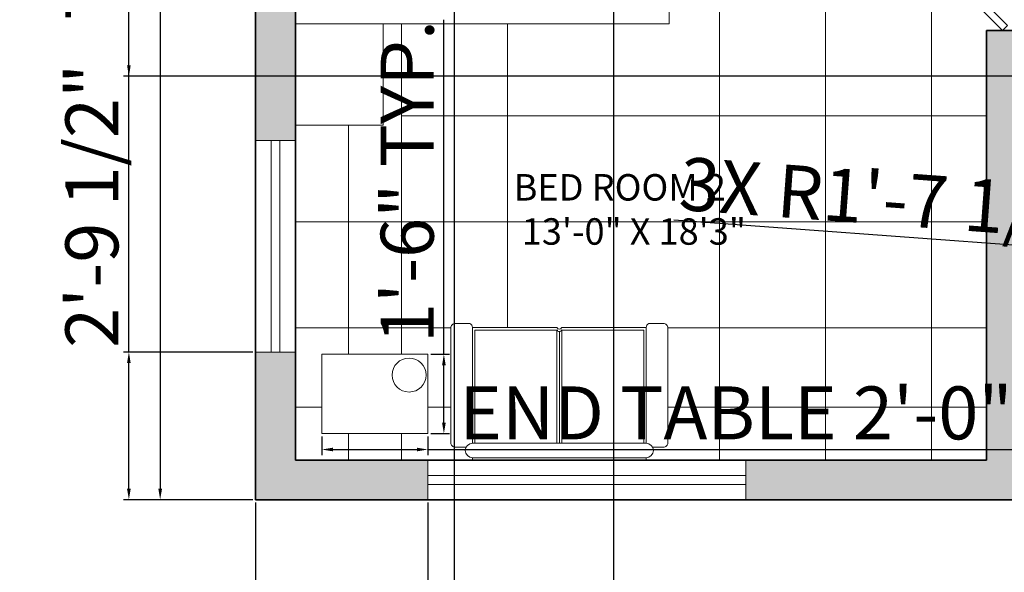
# Model space of a CAD drawing. Units: millimetres. Extents: x 542930 to 543750, y 628093 to 628738.
# Tile 2 of 14: x 542930 to 543153, y 628237 to 628363. Entities that reach past the tile are written whole.
import ezdxf

# ---------------------------------------------------------------- set-up
doc = ezdxf.new("R2010")
doc.units = ezdxf.units.MM
for name, color, linetype, lineweight in [('A-ANNO-DIMS', 2, 'Continuous', 18), ('A-FURN', 8, 'Continuous', 18), ('A-WALL', 7, 'Continuous', 35), ('DOORS', 30, 'Continuous', 18), ('WINDOW', 70, 'Continuous', 18)]:
    doc.layers.add(name, color=color, linetype=linetype, lineweight=lineweight)
for name, color, linetype, lineweight, true_color in [('A-AREA-IDEN', 40, 'Continuous', 18, 0xf8d731), ('A-FLOR-PATT', 241, 'Continuous', 13, 0xf7abae), ('A-WALL-PATT', 251, 'Continuous', 13, 0x636466)]:
    doc.layers.add(name, color=color, linetype=linetype, lineweight=lineweight, true_color=true_color)
doc.styles.get("Standard").update_dxf_attribs({"font": 'arial.ttf'})
doc.dimstyles.new('ISO-25', dxfattribs={"dimtxt": 12, "dimasz": 2.5, "dimexe": 1.25, "dimexo": 0.625, "dimtad": 1, "dimdec": 0, "dimlunit": 3, "dimtxsty": 'Standard', "dimcen": 2.5, "dimadec": 0, "dimazin": 0, "dimtfac": 1, "dimtdec": 0, "dimtmove": 0, "dimatfit": 3, "dimfxl": 1, "dimarcsym": 0})

# ---------------------------------------------------------------- blocks, each defined once
blk = doc.blocks.new('*U4')
for p, q in [((0, 0), (0, -6)), ((40, 0), (40, -6))]:
    blk.add_line(p, q)
blk.add_lwpolyline([(0, 0), (28.28, 28.28), (29.52, 27.05), (1.24, -1.24)], close=True)
blk.add_arc((0, 0), 40, 0, 45)
blk = doc.blocks.new('sofa')
for p, q in [((543001.62, 628230.38), (543001.62, 628182.38)), ((543010.62, 628230.38), (543045.62, 628230.38)), ((543045.62, 628229.38), (543045.62, 628182.38)), ((543046.62, 628228.78), (543046.62, 628182.38)), ((543091.62, 628230.38), (543091.62, 628182.38)), ((543010.62, 628176.38), (543082.62, 628176.38))]:
    blk.add_line(p, q)
for points in [[(543009.53, 628232.06), (543003.46, 628232.06, 0.414214), (543001.62, 628230.23)], [(543045.62, 628230.38, 0.623864), (543047.62, 628230.38), (543082.62, 628230.38), (543082.62, 628182.38), (543010.62, 628182.38), (543010.62, 628230.38, 0.297291), (543009.53, 628232.06)], [(543083.72, 628232.06, 0.297291), (543082.62, 628230.38), (543082.62, 628182.38)], [(543091.62, 628230.23, 0.414214), (543089.79, 628232.06), (543083.72, 628232.06)], [(543001.62, 628182.54, 0.414214), (543003.46, 628180.7), (543007.93, 628180.7)], [(543082.62, 628182.38, -1), (543082.62, 628176.38), (543082.62, 628175.38), (543010.62, 628175.38), (543010.62, 628176.38, -1), (543010.62, 628182.38)], [(543085.32, 628180.7), (543089.79, 628180.7, 0.414214), (543091.62, 628182.54)]]:
    blk.add_lwpolyline(points, format="xyb")
for points in [[(543011.62, 628182.38), (543011.62, 628229.38), (543045.62, 628229.38), (543045.62, 628229.4)], [(543047.62, 628182.38), (543047.62, 628229.38), (543047.62, 628229.4)], [(543047.62, 628229.38), (543081.62, 628229.38), (543081.62, 628182.38)]]:
    blk.add_lwpolyline(points)
blk.add_arc((543046.62, 628229.89), 1.11, 206.0829, 333.9171)
blk = doc.blocks.new('*D20')
at = {"layer": 'A-ANNO-DIMS', "color": 0, "lineweight": -2, "transparency": 16777216}
for p, q in [((542983.04, 628589.83), (542960.8, 628589.83)), ((542962.05, 628587.33), (542962.05, 628256.33)), ((542983.04, 628253.83), (542960.8, 628253.83))]:
    blk.add_line(p, q, dxfattribs=at)
at = {"layer": 'A-ANNO-DIMS', "color": 0, "transparency": 16777216}
for points in [[(542961.64, 628587.33), (542962.47, 628587.33), (542962.05, 628589.83)], [(542961.64, 628256.33), (542962.47, 628256.33), (542962.05, 628253.83)]]:
    blk.add_solid(points, dxfattribs=at)
at = {"layer": 'Defpoints', "color": 0, "transparency": 16777216}
for p in [(542983.67, 628589.83), (542962.05, 628253.83), (542983.67, 628253.83)]:
    blk.add_point(p, dxfattribs=at)
at = {"layer": 'A-ANNO-DIMS', "color": 0, "transparency": 16777216, "insert": (542955.3, 628421.83), "char_height": 12, "attachment_point": 5, "rotation": 90}
blk.add_mtext("28'", dxfattribs=at)
blk = doc.blocks.new('BEDROOM-END-TABLE')
for p, q in [((0, 0), (0, 18)), ((24.02, 18), (0, 18)), ((24.02, 0), (24.02, 18)), ((24.02, 0), (0, 0))]:
    blk.add_line(p, q)
blk.add_circle((19.74, 13.28), 3.85)
blk = doc.blocks.new('WIN-BEDROOM-FRONT')
for p, q in [((0, 9), (0, 0)), ((72, 9), (72, 0)), ((0, 5.5), (72, 5.5)), ((0, 3.5), (72, 3.5))]:
    blk.add_line(p, q)
blk = doc.blocks.new('WIN-BEDROOM-SIDE')
for p, q in [((0, 48), (9, 48)), ((3.5, 48), (3.5, 0)), ((5.5, 48), (5.5, 0)), ((0, 0), (9, 0))]:
    blk.add_line(p, q)
blk = doc.blocks.new('*D47')
at = {"layer": 'A-ANNO-DIMS', "color": 0, "lineweight": -2, "transparency": 16777216}
for p, q in [((542998.67, 628268.2), (542998.67, 628263.97)), ((543022.69, 628268.2), (543022.69, 628263.97)), ((543001.17, 628265.22), (543020.19, 628265.22)), ((543022.69, 628265.22), (543196.77, 628265.22))]:
    blk.add_line(p, q, dxfattribs=at)
at = {"layer": 'A-ANNO-DIMS', "color": 0, "transparency": 16777216}
for points in [[(543001.17, 628265.64), (543001.17, 628264.81), (542998.67, 628265.22)], [(543020.19, 628265.64), (543020.19, 628264.81), (543022.69, 628265.22)]]:
    blk.add_solid(points, dxfattribs=at)
at = {"layer": 'Defpoints', "color": 0, "transparency": 16777216}
for p in [(542998.67, 628268.83), (543022.69, 628268.83), (543022.69, 628265.22)]:
    blk.add_point(p, dxfattribs=at)
at = {"layer": 'A-ANNO-DIMS', "color": 0, "transparency": 16777216, "insert": (543110.98, 628271.97), "char_height": 12, "attachment_point": 5}
blk.add_mtext('END TABLE 2\'-0" TYP.', dxfattribs=at)
blk = doc.blocks.new('*D48')
at = {"layer": 'A-ANNO-DIMS', "color": 0, "lineweight": -2, "transparency": 16777216}
for p, q in [((543026.29, 628286.83), (543026.29, 628362.59)), ((543023.31, 628286.83), (543027.54, 628286.83)), ((543026.29, 628271.33), (543026.29, 628284.33)), ((543023.31, 628268.83), (543027.54, 628268.83))]:
    blk.add_line(p, q, dxfattribs=at)
at = {"layer": 'A-ANNO-DIMS', "color": 0, "transparency": 16777216}
for points in [[(543025.88, 628284.33), (543026.71, 628284.33), (543026.29, 628286.83)], [(543025.88, 628271.33), (543026.71, 628271.33), (543026.29, 628268.83)]]:
    blk.add_solid(points, dxfattribs=at)
at = {"layer": 'Defpoints', "color": 0, "transparency": 16777216}
for p in [(543022.69, 628286.83), (543026.29, 628286.83), (543022.69, 628268.83)]:
    blk.add_point(p, dxfattribs=at)
at = {"layer": 'A-ANNO-DIMS', "color": 0, "transparency": 16777216, "insert": (543019.54, 628325.96), "char_height": 12, "attachment_point": 5, "rotation": 90}
blk.add_mtext('1\'-6" TYP.', dxfattribs=at)
blk = doc.blocks.new('*D62')
at = {"layer": 'A-ANNO-DIMS', "color": 0, "lineweight": -2, "transparency": 16777216}
for p, q in [((542983.67, 628253.2), (542983.67, 628103.84)), ((543022.69, 628253.2), (543022.69, 628103.84)), ((542986.17, 628105.09), (543020.19, 628105.09))]:
    blk.add_line(p, q, dxfattribs=at)
at = {"layer": 'A-ANNO-DIMS', "color": 0, "transparency": 16777216}
for points in [[(542986.17, 628105.5), (542986.17, 628104.67), (542983.67, 628105.09)], [(543020.19, 628105.5), (543020.19, 628104.67), (543022.69, 628105.09)]]:
    blk.add_solid(points, dxfattribs=at)
at = {"layer": 'Defpoints', "color": 0, "transparency": 16777216}
for p in [(542983.67, 628253.83), (543022.69, 628253.83), (543022.69, 628105.09)]:
    blk.add_point(p, dxfattribs=at)
at = {"layer": 'A-ANNO-DIMS', "color": 0, "transparency": 16777216, "insert": (543003.18, 628111.84), "char_height": 12, "attachment_point": 5}
blk.add_mtext('3\'-3"', dxfattribs=at)
blk = doc.blocks.new('*D64')
at = {"layer": 'A-ANNO-DIMS', "color": 0, "lineweight": -2, "transparency": 16777216}
for p, q in [((542954.97, 628287.3), (542954.97, 628351.12)), ((542983.04, 628287.3), (542953.72, 628287.3)), ((542954.97, 628256.33), (542954.97, 628284.8)), ((542983.04, 628253.83), (542953.72, 628253.83))]:
    blk.add_line(p, q, dxfattribs=at)
at = {"layer": 'A-ANNO-DIMS', "color": 0, "transparency": 16777216}
for points in [[(542954.55, 628284.8), (542955.38, 628284.8), (542954.97, 628287.3)], [(542954.55, 628256.33), (542955.38, 628256.33), (542954.97, 628253.83)]]:
    blk.add_solid(points, dxfattribs=at)
at = {"layer": 'Defpoints', "color": 0, "transparency": 16777216}
for p in [(542954.97, 628287.3), (542983.67, 628287.3), (542983.67, 628253.83)]:
    blk.add_point(p, dxfattribs=at)
at = {"layer": 'A-ANNO-DIMS', "color": 0, "transparency": 16777216, "insert": (542948.14, 628320.46), "char_height": 12, "attachment_point": 5, "rotation": 90}
blk.add_mtext('2\'-9 1/2"', dxfattribs=at)
blk = doc.blocks.new('*D75')
at = {"layer": 'A-ANNO-DIMS', "color": 0, "lineweight": -2, "transparency": 16777216}
for p, q in [((543324.54, 628439.36), (542953.72, 628439.36)), ((542954.97, 628352.33), (542954.97, 628436.86)), ((543324.54, 628349.83), (542953.72, 628349.83))]:
    blk.add_line(p, q, dxfattribs=at)
at = {"layer": 'A-ANNO-DIMS', "color": 0, "transparency": 16777216}
for points in [[(542954.55, 628436.86), (542955.38, 628436.86), (542954.97, 628439.36)], [(542954.55, 628352.33), (542955.38, 628352.33), (542954.97, 628349.83)]]:
    blk.add_solid(points, dxfattribs=at)
at = {"layer": 'Defpoints', "color": 0, "transparency": 16777216}
for p in [(542954.97, 628439.36), (543325.17, 628439.36), (543325.17, 628349.83)]:
    blk.add_point(p, dxfattribs=at)
at = {"layer": 'A-ANNO-DIMS', "color": 0, "transparency": 16777216, "insert": (542948.14, 628394.6), "char_height": 12, "attachment_point": 5, "rotation": 90}
blk.add_mtext('7\'-5 1/2"', dxfattribs=at)
blk = doc.blocks.new('*D85')
at = {"layer": 'A-ANNO-DIMS', "color": 0, "lineweight": -2, "transparency": 16777216}
for p, q in [((543028.62, 628481.2), (543028.62, 628103.84)), ((543064.67, 628481.2), (543064.67, 628103.84)), ((543031.12, 628105.09), (543062.17, 628105.09))]:
    blk.add_line(p, q, dxfattribs=at)
at = {"layer": 'A-ANNO-DIMS', "color": 0, "transparency": 16777216}
for points in [[(543031.12, 628105.5), (543031.12, 628104.67), (543028.62, 628105.09)], [(543062.17, 628105.5), (543062.17, 628104.67), (543064.67, 628105.09)]]:
    blk.add_solid(points, dxfattribs=at)
at = {"layer": 'Defpoints', "color": 0, "transparency": 16777216}
for p in [(543028.62, 628481.83), (543064.67, 628481.83), (543064.67, 628105.09)]:
    blk.add_point(p, dxfattribs=at)
at = {"layer": 'A-ANNO-DIMS', "color": 0, "transparency": 16777216, "insert": (543046.65, 628111.84), "char_height": 12, "attachment_point": 5}
blk.add_mtext('3\'-0"', dxfattribs=at)
blk = doc.blocks.new('*D93')
at = {"layer": 'A-ANNO-DIMS', "color": 0, "lineweight": -2, "transparency": 16777216}
for p, q in [((543078.39, 628317.26), (543178.99, 628309.88)), ((543200.81, 628308.28), (543181.49, 628309.7))]:
    blk.add_line(p, q, dxfattribs=at)
at = {"layer": 'A-ANNO-DIMS', "color": 0, "transparency": 16777216}
blk.add_solid([(543179.02, 628310.3), (543178.96, 628309.46), (543181.49, 628309.7)], dxfattribs=at)
at = {"layer": 'Defpoints', "color": 0, "transparency": 16777216}
for p in [(543181.49, 628309.7), (543200.81, 628308.28)]:
    blk.add_point(p, dxfattribs=at)
at = {"layer": 'A-ANNO-DIMS', "color": 0, "transparency": 16777216, "insert": (543127.94, 628320.48), "char_height": 12, "attachment_point": 5, "rotation": 355.8053}
blk.add_mtext('3X R1\'-7 1/2"', dxfattribs=at)
blk = doc.blocks.new('*D94')
at = {"layer": 'A-ANNO-DIMS', "color": 0, "lineweight": -2, "transparency": 16777216}
for p, q in [((543143.96, 628391.37), (543186.37, 628329.39)), ((543198.34, 628311.9), (543187.78, 628327.33))]:
    blk.add_line(p, q, dxfattribs=at)
at = {"layer": 'A-ANNO-DIMS', "color": 0, "transparency": 16777216}
blk.add_solid([(543186.71, 628329.63), (543186.02, 628329.15), (543187.78, 628327.33)], dxfattribs=at)
at = {"layer": 'Defpoints', "color": 0, "transparency": 16777216}
for p in [(543187.78, 628327.33), (543198.34, 628311.9)]:
    blk.add_point(p, dxfattribs=at)
at = {"layer": 'A-ANNO-DIMS', "color": 0, "transparency": 16777216, "insert": (543170.1, 628365.27), "char_height": 12, "attachment_point": 5, "rotation": 304.3793}
blk.add_mtext('R1\'-6 1/2"', dxfattribs=at)
blk = doc.blocks.new('*D95')
at = {"layer": 'A-ANNO-DIMS', "color": 0, "lineweight": -2, "transparency": 16777216}
for p, q in [((543144.53, 628390.54), (543186.93, 628328.57)), ((543198.34, 628311.9), (543188.34, 628326.5))]:
    blk.add_line(p, q, dxfattribs=at)
at = {"layer": 'A-ANNO-DIMS', "color": 0, "transparency": 16777216}
blk.add_solid([(543187.28, 628328.8), (543186.59, 628328.33), (543188.34, 628326.5)], dxfattribs=at)
at = {"layer": 'Defpoints', "color": 0, "transparency": 16777216}
for p in [(543188.34, 628326.5), (543198.34, 628311.9)]:
    blk.add_point(p, dxfattribs=at)
at = {"layer": 'A-ANNO-DIMS', "color": 0, "transparency": 16777216, "insert": (543170.66, 628364.44), "char_height": 12, "attachment_point": 5, "rotation": 304.3778}
blk.add_mtext('R1\'-5 1/2"', dxfattribs=at)

msp = doc.modelspace()

# ---------------------------------------------------------------- hatches: boundary and pattern name
at = {"layer": 'A-WALL-PATT'}
h = msp.add_hatch(color=256, dxfattribs=at)
h.dxf.hatch_style = 1
h.paths.add_polyline_path([(542992.67, 628481.83), (543028.62, 628481.83), (543028.62, 628490.83), (542992.67, 628490.83), (542992.67, 628580.83), (543113.07, 628580.83), (543113.07, 628589.83), (542983.67, 628589.83), (542983.67, 628335.3), (542992.67, 628335.3)])
h = msp.add_hatch(color=256, dxfattribs=at)
h.dxf.hatch_style = 1
h.paths.add_polyline_path([(543158.17, 628340.83), (543205.67, 628340.83), (543205.67, 628349.83), (543158.17, 628349.83), (543158.17, 628360.23), (543149.17, 628360.23), (543149.17, 628262.83), (543094.69, 628262.83), (543094.69, 628253.83), (543158.17, 628253.83)])
h = msp.add_hatch(color=256, dxfattribs=at)
h.dxf.hatch_style = 1
h.paths.add_polyline_path([(543022.69, 628262.83), (542992.67, 628262.83), (542992.67, 628287.3), (542983.67, 628287.3), (542983.67, 628253.83), (543022.69, 628253.83)])

# ---------------------------------------------------------------- linework, layer by layer
at = {"layer": 'A-FLOR-PATT'}
for p, q in [((543088.67, 628262.83), (543088.67, 628456.83)), ((543112.67, 628262.83), (543112.67, 628456.83)), ((543136.67, 628262.83), (543136.67, 628456.83)), ((543016.67, 628286.83), (543016.67, 628361.72)), ((543040.67, 628292.83), (543040.67, 628361.72)), ((543064.67, 628292.83), (543064.67, 628361.72)), ((543016.67, 628340.83), (543149.17, 628340.83)), ((543004.67, 628286.83), (543004.67, 628338.72)), ((542992.67, 628316.83), (543149.17, 628316.83)), ((542992.67, 628292.83), (543027.87, 628292.83)), ((543077.01, 628292.83), (543149.17, 628292.83)), ((542992.67, 628274.83), (542998.67, 628274.83)), ((543022.69, 628274.83), (543027.87, 628274.83)), ((543077.01, 628274.83), (543149.17, 628274.83)), ((543004.67, 628262.83), (543004.67, 628268.83)), ((543016.67, 628262.83), (543016.67, 628268.83))]:
    msp.add_line(p, q, dxfattribs=at)
at = {"layer": 'A-FURN'}
for p, q in [((543077.27, 628424.17), (543077.27, 628361.72)), ((543077.27, 628361.72), (542992.67, 628361.72)), ((543012.52, 628361.72), (543012.52, 628338.72)), ((543012.52, 628338.72), (542992.67, 628338.72))]:
    msp.add_line(p, q, dxfattribs=at)
at = {"layer": 'A-WALL'}
for p, q in [((542992.67, 628262.83), (542992.67, 628481.83)), ((543149.17, 628262.83), (543149.17, 628360.23)), ((543158.17, 628360.23), (543149.17, 628360.23)), ((543149.17, 628262.83), (542992.67, 628262.83))]:
    msp.add_line(p, q, dxfattribs=at)
msp.add_lwpolyline([(543499.67, 628253.83), (542983.67, 628253.83), (542983.67, 628589.83)], dxfattribs=at)

# ---------------------------------------------------------------- block references
at = {"layer": 'A-FURN', "xscale": 0.5460747824189197, "yscale": 0.5460747824189197, "zscale": 0.5460747824189197}
msp.add_blockref('sofa', (246508.37, 285232.09), dxfattribs=at)
at = {"layer": 'A-FURN'}
msp.add_blockref('BEDROOM-END-TABLE', (542998.67, 628268.83), dxfattribs=at)
at = {"layer": 'DOORS', "xscale": 0.9000000000029102, "yscale": 0.9000000000029102, "zscale": 0.9000000000029102, "rotation": 90}
msp.add_blockref('*U4', (543152.77, 628360.23), dxfattribs=at)
at = {"layer": 'WINDOW'}
for name, p in [('WIN-BEDROOM-SIDE', (542983.67, 628287.3)), ('WIN-BEDROOM-FRONT', (543022.69, 628253.83))]:
    msp.add_blockref(name, p, dxfattribs=at)

# ---------------------------------------------------------------- texts
at = {"layer": 'A-AREA-IDEN', "insert": (543038.43, 628327.65), "char_height": 6, "attachment_point": 1}
msp.add_mtext_dynamic_manual_height_columns('  BED ROOM 2\\P   13\'-0" X 18\'3"', width=63.3037, gutter_width=12.5, heights=[0], dxfattribs=at)

# ---------------------------------------------------------------- dimensions: what is measured, and where the dimension line sits
at = {"layer": 'A-ANNO-DIMS'}
for base, p1, p2, override, picture, middle in [((542962.05, 628253.83), (542983.67, 628589.83), (542983.67, 628253.83), {"dimclrd": 0, "dimclre": 0, "dimclrt": 0}, '*D20', (542955.3, 628421.83)), ((542954.97, 628439.36), (543325.17, 628349.83), (543325.17, 628439.36), {"dimdec": 1, "dimlfac": 1, "dimrnd": 0, "dimzin": 1, "dimdsep": 46, "dimlunit": 4, "dimfrac": 2}, '*D75', (542948.14, 628394.6)), ((542954.97, 628287.3), (542983.67, 628253.83), (542983.67, 628287.3), {"dimdec": 1, "dimlfac": 1, "dimrnd": 0, "dimzin": 1, "dimdsep": 46, "dimlunit": 4, "dimfrac": 2}, '*D64', (542948.14, 628320.46))]:
    dim = msp.add_linear_dim(base=base, p1=p1, p2=p2, angle=90, dimstyle='ISO-25', override=override, dxfattribs=at)
    dim.commit()
    dim.dimension.update_dxf_attribs({"geometry": picture, "text_midpoint": middle})
for base, p1, p2, picture, middle in [((543064.6669, 628105.0858), (543028.6237, 628481.8258), (543064.6669, 628481.8258), '*D85', (543046.6453, 628111.8418)), ((543022.69, 628105.09), (542983.67, 628253.83), (543022.69, 628253.83), '*D62', (543003.18, 628111.84))]:
    dim = msp.add_linear_dim(base=base, p1=p1, p2=p2, dimstyle='ISO-25', override={"dimdec": 1, "dimlfac": 1, "dimrnd": 0, "dimzin": 1, "dimdsep": 46, "dimlunit": 4, "dimfrac": 2}, dxfattribs=at)
    dim.commit()
    dim.dimension.update_dxf_attribs({"geometry": picture, "text_midpoint": middle})
for mpoint, picture, middle in [((543187.78, 628327.33), '*D94', (543170.1, 628365.27)), ((543188.34, 628326.5), '*D95', (543170.66, 628364.44))]:
    dim = msp.add_radius_dim(center=(543198.34, 628311.9), mpoint=mpoint, dimstyle='ISO-25', override={"dimdec": 1, "dimlfac": 1, "dimrnd": 0, "dimzin": 1, "dimdsep": 46, "dimlunit": 4, "dimfrac": 2}, dxfattribs=at)
    dim.commit()
    dim.dimension.update_dxf_attribs({"geometry": picture, "text_midpoint": middle})
dim = msp.add_linear_dim(base=(543026.29, 628286.83), p1=(543022.69, 628268.83), p2=(543022.69, 628286.83), angle=90, text='<> TYP.', dimstyle='ISO-25', override={"dimdec": 1, "dimlfac": 1, "dimrnd": 0, "dimzin": 1, "dimdsep": 46, "dimlunit": 4, "dimfrac": 2}, dxfattribs=at)
dim.commit()
dim.dimension.update_dxf_attribs({"geometry": '*D48', "text_midpoint": (543019.54, 628325.96)})
dim = msp.add_radius_dim(center=(543200.81, 628308.28), mpoint=(543181.49, 628309.7), text='3X <>', dimstyle='ISO-25', override={"dimdec": 1, "dimlfac": 1, "dimrnd": 0, "dimzin": 1, "dimdsep": 46, "dimlunit": 4, "dimfrac": 2}, dxfattribs=at)
dim.commit()
dim.dimension.update_dxf_attribs({"geometry": '*D93', "text_midpoint": (543127.94, 628320.48)})
dim = msp.add_linear_dim(base=(543022.69, 628265.22), p1=(542998.67, 628268.83), p2=(543022.69, 628268.83), text='END TABLE <> TYP.', dimstyle='ISO-25', override={"dimdec": 1, "dimlfac": 1, "dimrnd": 0, "dimzin": 1, "dimdsep": 46, "dimlunit": 4, "dimfrac": 2}, dxfattribs=at)
dim.commit()
dim.dimension.update_dxf_attribs({"geometry": '*D47', "text_midpoint": (543110.98, 628271.97)})

doc.saveas('drawing.dxf')
